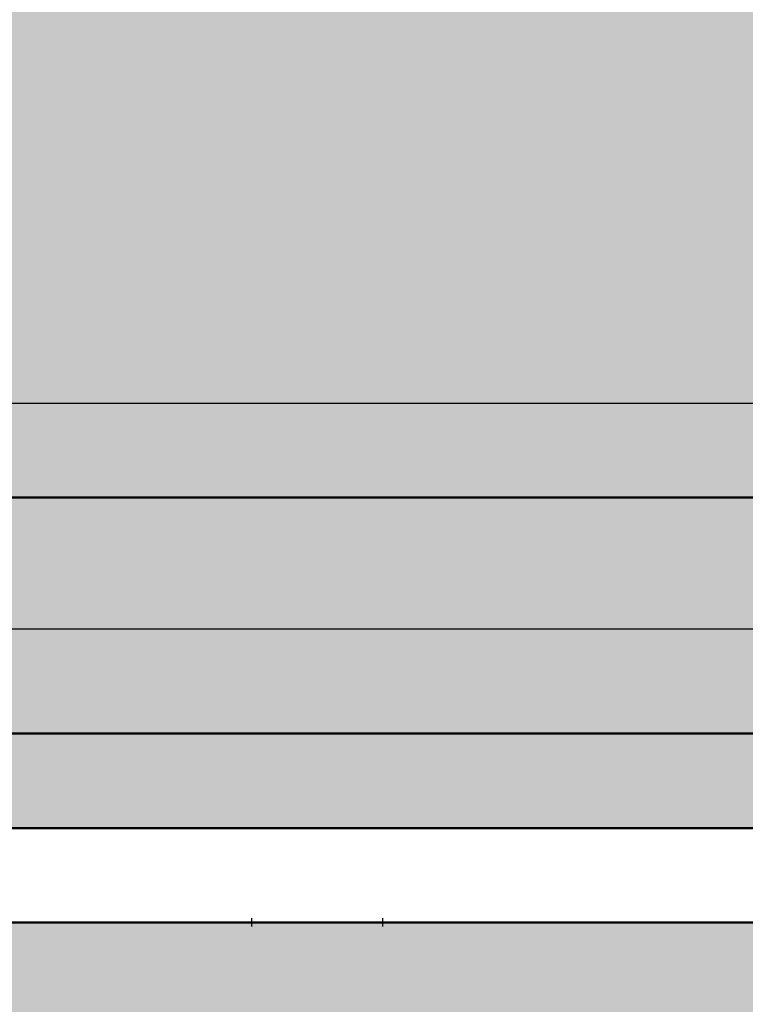
# Model space of a CAD drawing. Units: inches. Extents: x -12 to 334, y -10 to 186.
# Tile 46 of 77: x 182.48 to 197.85, y 90.16 to 111.02. Entities that reach past the tile are written whole.
import ezdxf

# ---------------------------------------------------------------- set-up
doc = ezdxf.new("R2010")
doc.units = ezdxf.units.IN
doc.header["$MEASUREMENT"] = 0
for name, color, linetype, lineweight in [('M-DIMS', 2, 'Continuous', 18), ('M-EQPM', 7, 'Continuous', 50), ('M-EQPM-PATT', 8, 'Continuous', 18)]:
    doc.layers.add(name, color=color, linetype=linetype, lineweight=lineweight)
doc.styles.get("Standard").update_dxf_attribs({"font": 'arial.ttf'})
doc.dimstyles.get("Standard").update_dxf_attribs({"dimtxt": 0.18, "dimasz": 0.18, "dimexe": 0.18, "dimexo": 0.0625, "dimgap": 0.09, "dimtad": 0, "dimtih": 1, "dimtoh": 1, "dimdec": 4, "dimzin": 0, "dimdsep": 46, "dimtxsty": 'Standard', "dimcen": 0.09, "dimadec": 0, "dimazin": 0, "dimtfac": 1, "dimtdec": 4, "dimtofl": 0, "dimtmove": 0, "dimatfit": 3, "dimfxl": 1, "dimtolj": 1, "dimtzin": 0, "dimarcsym": 0})

# ---------------------------------------------------------------- blocks, each defined once
blk = doc.blocks.new('*D1')
at = {"layer": 'Defpoints', "color": 0, "transparency": 16777216}
for p in [(281.426, 91.899), (3.376, 80.692), (281.426, 14.304)]:
    blk.add_point(p, dxfattribs=at)
at = {"layer": 'M-DIMS', "color": 0, "lineweight": -2, "transparency": 16777216}
for p, q in [((281.426, 91.836), (281.426, 14.124)), ((3.376, 80.629), (3.376, 14.124)), ((3.556, 14.304), (141.935, 14.304)), ((281.246, 14.304), (142.867, 14.304))]:
    blk.add_line(p, q, dxfattribs=at)
at = {"layer": 'M-DIMS', "color": 0, "transparency": 16777216}
for points in [[(3.556, 14.334), (3.556, 14.274), (3.376, 14.304)], [(281.246, 14.334), (281.246, 14.274), (281.426, 14.304)]]:
    blk.add_solid(points, dxfattribs=at)
at = {"layer": 'M-DIMS', "color": 0, "transparency": 16777216, "insert": (142.401, 14.304), "char_height": 0.18, "attachment_point": 5}
blk.add_mtext('\\A1;278.05', dxfattribs=at)
blk = doc.blocks.new('*D17')
at = {"layer": 'Defpoints', "color": 0, "transparency": 16777216}
for p in [(106.177, 102.896), (105.892, 56.321), (295.976, 56.321)]:
    blk.add_point(p, dxfattribs=at)
at = {"layer": 'M-DIMS', "color": 0, "lineweight": -2, "transparency": 16777216}
for p, q in [((106.24, 102.896), (296.156, 102.896)), ((295.976, 102.716), (295.976, 79.79)), ((295.976, 56.501), (295.976, 79.426)), ((105.954, 56.321), (296.156, 56.321))]:
    blk.add_line(p, q, dxfattribs=at)
at = {"layer": 'M-DIMS', "color": 0, "transparency": 16777216}
for points in [[(295.946, 102.716), (296.006, 102.716), (295.976, 102.896)], [(295.946, 56.501), (296.006, 56.501), (295.976, 56.321)]]:
    blk.add_solid(points, dxfattribs=at)
at = {"layer": 'M-DIMS', "color": 0, "transparency": 16777216, "insert": (295.976, 79.608), "char_height": 0.18, "attachment_point": 5}
blk.add_mtext('\\A1;46.575', dxfattribs=at)
blk = doc.blocks.new('*D35')
at = {"layer": 'Defpoints', "color": 0, "transparency": 16777216}
for p in [(216.428, 98.108), (-11.174, 61.105), (216.428, 61.105)]:
    blk.add_point(p, dxfattribs=at)
at = {"layer": 'M-DIMS', "color": 0, "lineweight": -2, "transparency": 16777216}
for p, q in [((216.365, 98.108), (-11.354, 98.108)), ((-11.174, 97.928), (-11.174, 79.788)), ((-11.174, 61.285), (-11.174, 79.424)), ((216.365, 61.105), (-11.354, 61.105))]:
    blk.add_line(p, q, dxfattribs=at)
at = {"layer": 'M-DIMS', "color": 0, "transparency": 16777216}
for points in [[(-11.204, 97.928), (-11.144, 97.928), (-11.174, 98.108)], [(-11.204, 61.285), (-11.144, 61.285), (-11.174, 61.105)]]:
    blk.add_solid(points, dxfattribs=at)
at = {"layer": 'M-DIMS', "color": 0, "transparency": 16777216, "insert": (-11.174, 79.606), "char_height": 0.18, "attachment_point": 5}
blk.add_mtext('\\A1;37', dxfattribs=at)
blk = doc.blocks.new('*D40')
at = {"layer": 'Defpoints', "color": 0, "transparency": 16777216}
for p in [(278.229, 116.208), (187.394, 91.899)]:
    blk.add_point(p, dxfattribs=at)
at = {"layer": 'M-DIMS', "color": 0, "lineweight": -2, "transparency": 16777216}
for p, q in [((332.73, 130.793), (278.403, 116.254)), ((187.394, 91.809), (187.394, 91.989)), ((187.304, 91.899), (187.484, 91.899))]:
    blk.add_line(p, q, dxfattribs=at)
at = {"layer": 'M-DIMS', "color": 0, "transparency": 16777216}
blk.add_solid([(278.395, 116.283), (278.411, 116.225), (278.229, 116.208)], dxfattribs=at)
at = {"layer": 'M-DIMS', "color": 0, "transparency": 16777216, "insert": (333.21, 130.793), "char_height": 0.18, "attachment_point": 5}
blk.add_mtext('\\A1;R94.03', dxfattribs=at)
blk = doc.blocks.new('*D41')
at = {"layer": 'Defpoints', "color": 0, "transparency": 16777216}
for p in [(190.169, 91.899), (277.343, 68.515)]:
    blk.add_point(p, dxfattribs=at)
at = {"layer": 'M-DIMS', "color": 0, "lineweight": -2, "transparency": 16777216}
for p, q in [((190.169, 91.809), (190.169, 91.989)), ((190.079, 91.899), (190.259, 91.899)), ((329.648, 54.485), (277.517, 68.469)), ((329.828, 54.485), (329.648, 54.485))]:
    blk.add_line(p, q, dxfattribs=at)
at = {"layer": 'M-DIMS', "color": 0, "transparency": 16777216}
blk.add_solid([(277.525, 68.498), (277.509, 68.44), (277.343, 68.515)], dxfattribs=at)
at = {"layer": 'M-DIMS', "color": 0, "transparency": 16777216, "insert": (330.307, 54.485), "char_height": 0.18, "attachment_point": 5}
blk.add_mtext('\\A1;R90.26', dxfattribs=at)

msp = doc.modelspace()

# ---------------------------------------------------------------- hatches: boundary and pattern name
at = {"layer": 'M-EQPM-PATT', "transparency": 33554556}
h = msp.add_hatch(color=256, dxfattribs=at)
h.set_gradient(color1=(248, 206, 179), color2=(248, 206, 179), tint=1)
h.paths.add_polyline_path([(179.7818, 136.8871), (126.9567, 136.8871), (106.1771, 100.8958), (171.5458, 100.8958)])
h.paths.add_polyline_path([(268.3808, 136.9435), (214.0166, 136.9435), (214.0166, 154.8345), (196.3421, 154.8345), (196.3421, 136.8871), (179.7818, 136.8871), (171.5458, 100.8958), (231.7758, 100.8958, -0.4142136), (251.9801, 80.6915), (279.7263, 80.6915, 0.1631825)])
at = {"layer": 'M-EQPM-PATT'}
h = msp.add_hatch(color=256, dxfattribs=at)
h.set_gradient(color1=(205, 32, 39), color2=(205, 32, 39), tint=1)
h.paths.add_polyline_path([(64.5, 80.754), (64.5, 89.8963), (226.6083, 89.8963, -1), (226.6083, 69.6117), (64.5, 69.6117), (64.5, 78.754), (4.4744, 78.754, 0.384914), (23.5807, 61.4872), (37.1002, 61.4872), (37.1002, 33.6752), (53.1002, 33.6752), (53.1002, 61.4872), (64.5, 61.4872), (64.5, 63.6117), (226.6083, 63.6117, 1), (226.6083, 95.8963), (64.5, 95.8963), (64.5, 99.8958), (53.1002, 99.8958), (53.1002, 127.7078), (37.1002, 127.7078), (37.1002, 99.8958), (23.5807, 99.8958, 0.4132606), (4.3766, 80.754)])
h.paths.add_polyline_path([(64.5, 91.8963), (64.5, 93.8963), (226.6083, 93.8963, -1), (226.6083, 65.6117), (64.5, 65.6117), (64.5, 67.6117), (226.6083, 67.6117, 1), (226.6083, 91.8963)], flags=16)
h = msp.add_hatch(color=256, dxfattribs=at)
h.set_gradient(color1=(94, 103, 175), color2=(94, 103, 175), tint=1)
h.paths.add_polyline_path([(129.093, 89.8963), (86.8879, 89.8963), (86.8879, 69.6117), (129.093, 69.6117)], flags=17)
h.paths.add_polyline_path([(170.9079, 89.8963), (130.8573, 89.8963), (130.8573, 69.6117), (170.9079, 69.6117)], flags=17)
h.paths.add_polyline_path([(216.4278, 89.8963), (172.6722, 89.8963), (172.6722, 69.6117), (216.4278, 69.6117)], flags=17)
h.paths.add_polyline_path([(245.9354, 82.6969), (247.9354, 82.6969), (247.9354, 46.8541), (268.3808, 46.8541, 0.0998398), (279.7263, 80.6915), (251.9801, 80.6915, 0.4142136), (231.7758, 100.8958), (84.7229, 100.8958), (84.7229, 109.0583), (83.7229, 109.0583), (83.7229, 95.8963), (129.093, 95.8963), (129.093, 98.1081), (130.8573, 98.1081), (130.8573, 95.8963), (170.9079, 95.8963), (170.9079, 98.1081), (172.6722, 98.1081), (172.6722, 95.8963), (216.4278, 95.8963), (216.4278, 98.1081), (218.1922, 98.1081), (218.1922, 95.8963), (226.6083, 95.8963, -1), (226.6083, 63.6117), (218.1922, 63.6117), (218.1922, 61.1045), (216.4278, 61.1045), (216.4278, 63.6117), (172.6722, 63.6117), (172.6722, 61.1045), (170.9079, 61.1045), (170.9079, 63.6117), (130.8573, 63.6117), (130.8573, 61.1045), (129.093, 61.1045), (129.093, 63.6117), (87.8879, 63.6117), (87.8879, 56.3205), (105.8919, 56.3205), (105.8919, 28.8541), (115.8919, 28.8541), (115.8919, 46.8541), (222.5761, 46.8541), (222.5761, 30.8541), (232.5761, 30.8541), (232.5761, 46.8541), (245.9354, 46.8541)])
h.paths.add_polyline_path([(86.8879, 89.8963), (75.9244, 89.8963), (75.9244, 69.6117), (86.8879, 69.6117)])
h.paths.add_polyline_path([(83.7229, 109.0583), (75.9244, 109.0583), (75.9244, 95.8963), (83.7229, 95.8963)])
h.paths.add_polyline_path([(226.6083, 89.8963), (218.1922, 89.8963), (218.1922, 69.6117), (226.6083, 69.6117, 1)], flags=17)
h = msp.add_hatch(color=256, dxfattribs=at)
h.set_gradient(color1=(0, 0, 255), color2=(0, 0, 255), tint=1)
h.paths.add_polyline_path([(84.7229, 100.8958), (84.7229, 109.0583), (83.7229, 109.0583), (83.7229, 95.8963), (129.093, 95.8963), (129.093, 98.1081), (130.8573, 98.1081), (130.8573, 95.8963), (170.9079, 95.8963), (170.9079, 98.1081), (172.6722, 98.1081), (172.6722, 95.8963), (216.4278, 95.8963), (216.4278, 98.1081), (218.1922, 98.1081), (218.1922, 95.8963), (226.6083, 95.8963, -1), (226.6083, 63.6117), (218.1922, 63.6117), (218.1922, 61.1045), (216.4278, 61.1045), (216.4278, 63.6117), (172.6722, 63.6117), (172.6722, 61.1045), (170.9079, 61.1045), (170.9079, 63.6117), (130.8573, 63.6117), (130.8573, 61.1045), (129.093, 61.1045), (129.093, 63.6117), (87.8879, 63.6117), (87.8879, 56.3205), (105.8919, 56.3205), (105.8919, 28.8541), (115.8919, 28.8541), (115.8919, 46.8541), (222.5761, 46.8541), (222.5761, 30.8541), (232.5761, 30.8541), (232.5761, 46.8541), (245.9354, 46.8541), (245.9354, 82.6969), (247.9354, 82.6969), (247.9354, 46.8541), (268.3808, 46.8541, 0.0998398), (279.7263, 80.6915), (251.9801, 80.6915, 0.4142136), (231.7758, 100.8958)])

# ---------------------------------------------------------------- linework, layer by layer
at = {"layer": 'M-EQPM'}
msp.add_lwpolyline([(84.7229, 100.8958), (231.7758, 100.8958)], dxfattribs=at)
for points in [[(64.5, 63.6117), (226.6083, 63.6117, 1), (226.6083, 95.8963), (64.5, 95.8963)], [(64.5, 65.6117), (226.6083, 65.6117, 1), (226.6083, 93.8963), (64.5, 93.8963)], [(64.5, 67.6117), (226.6083, 67.6117, 1), (226.6083, 91.8963), (64.5, 91.8963)]]:
    msp.add_lwpolyline(points, format="xyb", dxfattribs=at)

# ---------------------------------------------------------------- dimensions: what is measured, and where the dimension line sits
at = {"layer": 'M-DIMS'}
for center, mpoint, picture, middle in [((187.3936, 91.8988), (278.2291, 116.2078), '*D40', (332.7304, 130.7932)), ((190.1689, 91.8988), (277.3431, 68.5153), '*D41', (330.3074, 54.4851))]:
    dim = msp.add_radius_dim(center=center, mpoint=mpoint, dimstyle='Standard', override={"dimdec": 2, "dimlfac": 1, "dimrnd": 0, "dimzin": 0, "dimdsep": 46, "dimlunit": 2}, dxfattribs=at)
    dim.commit()
    dim.dimension.update_dxf_attribs({"geometry": picture, "text_midpoint": middle, "dimtype": 164})
for base, p1, p2, override, picture, middle in [((295.9756, 56.3205), (106.1771, 102.8958), (105.8919, 56.3205), {"dimdec": 3, "dimlfac": 1, "dimrnd": 0, "dimzin": 0, "dimdsep": 46, "dimlunit": 2}, '*D17', (295.9756, 79.6082)), ((-11.1736, 61.1045), (216.4278, 98.1081), (216.4278, 61.1045), {"dimdec": 0, "dimlfac": 1, "dimrnd": 0, "dimzin": 0, "dimdsep": 46, "dimlunit": 2}, '*D35', (-11.1735, 79.6063))]:
    dim = msp.add_linear_dim(base=base, p1=p1, p2=p2, angle=90, dimstyle='Standard', override=override, dxfattribs=at)
    dim.commit()
    dim.dimension.update_dxf_attribs({"geometry": picture, "text_midpoint": middle})
dim = msp.add_linear_dim(base=(281.4256, 14.3041), p1=(3.3765, 80.6915), p2=(281.4256, 91.8988), dimstyle='Standard', override={"dimdec": 2, "dimlfac": 1, "dimrnd": 0, "dimzin": 0, "dimdsep": 46, "dimlunit": 2}, dxfattribs=at)
dim.commit()
dim.dimension.update_dxf_attribs({"geometry": '*D1', "text_midpoint": (142.401, 14.3041)})

doc.saveas('drawing.dxf')
